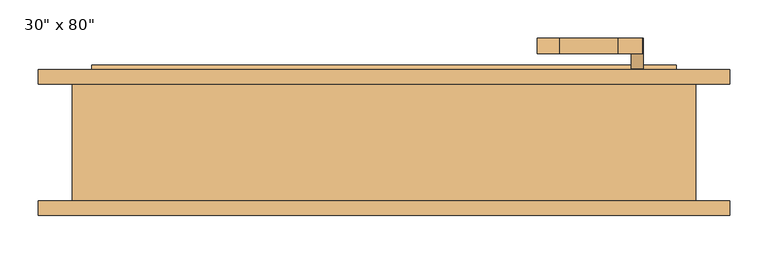
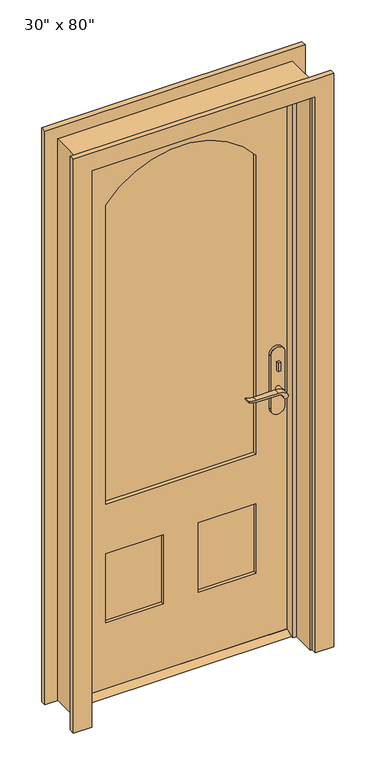
"""IFC4 building model written with IfcOpenShell, lengths in millimetres: door geometry."""

from ifc_helpers import new_model, si_unit, point, frame, frame_2d, origin, place, context, project, spatial, polyline, circle_curve, trimmed, segment, composite_curve, outline, extrude, faceted_brep, source, transform, mapped, element, save


def door_14b9be53(model_context):
    return source(origin(), model_context, "Body", "SolidModel", [
        extrude(outline(polyline([(38.1, 12.7), (73.025, 12.7), (98.425, 0.0), (12.7, 0.0), (38.1, 12.7)])), frame((-381.0, 0.0, 0.0), z_axis=(1.0, 0.0, 0.0), x_axis=(0.0, 1.0, 0.0)), (0.0, 0.0, 1.0), 762.0),
        extrude(outline(polyline([(335.2, 18.1), (325.2, 18.1), (325.2, 28.1), (335.2, 28.1), (335.2, 18.1)])), frame((0.0, 0.0, 981.9), z_axis=(0.0, 0.0, 1.0), x_axis=(1.0, 0.0, 0.0)), (0.0, 0.0, 1.0), 30.0),
        extrude(outline(composite_curve([segment(trimmed(circle_curve(frame_2d((996.9, 330.2)), 8.0), [point((996.9, 322.2))], [point((996.9, 338.2))], False, "CARTESIAN"), True, "CONTINUOUS"), segment(trimmed(circle_curve(frame_2d((996.9, 330.2)), 8.0), [point((996.9, 338.2))], [point((996.9, 322.2))], False, "CARTESIAN"), True, "CONTINUOUS")], self_intersect=False)), frame((0.0, 83.025, 0.0), z_axis=(0.0, 1.0, 0.0), x_axis=(0.0, 0.0, 1.0)), (0.0, 0.0, 1.0), 10.0),
        extrude(outline(composite_curve([segment(trimmed(circle_curve(frame_2d((897.1555521, 306.5324871)), 37.2832219), [point((919.0523287, 336.7081363))], [point((934.4, 304.8325667))], False, "CARTESIAN"), True, "CONTINUOUS"), segment(polyline([(934.4, 304.8325667), (934.4, 228.5564091)]), True, "CONTINUOUS"), segment(trimmed(circle_curve(frame_2d((1017.6850638, 228.6227909)), 83.2850902), [point((934.4, 228.5564091))], [point((939.4, 200.2))], True, "CARTESIAN"), True, "CONTINUOUS"), segment(polyline([(939.4, 200.2), (936.6135558, 200.2)]), True, "CONTINUOUS"), segment(trimmed(circle_curve(frame_2d((986.6709207, 232.1396612)), 59.3791355), [point((936.6135558, 200.2))], [point((927.4, 228.5564091))], False, "CARTESIAN"), True, "CONTINUOUS"), segment(polyline([(927.4, 228.5564091), (927.4, 304.8138099)]), True, "CONTINUOUS"), segment(trimmed(circle_curve(frame_2d((909.2738613, 304.8138099)), 18.1261387), [point((927.4, 304.8138099))], [point((914.4, 322.2))], True, "CARTESIAN"), True, "CONTINUOUS"), segment(trimmed(circle_curve(frame_2d((914.4, 330.2)), 8.0), [point((914.4, 322.2))], [point((919.0523287, 336.7081363))], False, "CARTESIAN"), True, "CONTINUOUS")], self_intersect=False)), frame((0.0, -21.9, 0.0), z_axis=(0.0, 1.0, 0.0), x_axis=(0.0, 0.0, 1.0)), (0.0, 0.0, 1.0), 20.0),
        extrude(outline(composite_curve([segment(trimmed(circle_curve(frame_2d((914.4, 330.2)), 8.0), [point((914.3999903, 322.2))], [point((919.0523287, 336.7081363))], False, "CARTESIAN"), True, "CONTINUOUS"), segment(trimmed(circle_curve(frame_2d((897.1555521, 306.5324871)), 37.2832219), [point((919.0523287, 336.7081363))], [point((934.4, 304.8325667))], False, "CARTESIAN"), True, "CONTINUOUS"), segment(polyline([(934.4, 304.8325667), (934.4, 228.5564091)]), True, "CONTINUOUS"), segment(trimmed(circle_curve(frame_2d((1017.6850638, 228.6227909)), 83.2850902), [point((934.4, 228.5564091))], [point((939.4, 200.2))], True, "CARTESIAN"), True, "CONTINUOUS"), segment(polyline([(939.4, 200.2), (936.6135558, 200.2)]), True, "CONTINUOUS"), segment(trimmed(circle_curve(frame_2d((986.6709207, 232.1396612)), 59.3791355), [point((936.6135558, 200.2))], [point((927.4, 228.5564091))], False, "CARTESIAN"), True, "CONTINUOUS"), segment(polyline([(927.4, 228.5564091), (927.4, 304.8138122)]), True, "CONTINUOUS"), segment(trimmed(circle_curve(frame_2d((909.2738682, 304.8138122)), 18.1261318), [point((927.4, 304.8138122))], [point((914.3999903, 322.2))], True, "CARTESIAN"), True, "CONTINUOUS")], self_intersect=False)), frame((0.0, 113.025, 0.0), z_axis=(0.0, 1.0, 0.0), x_axis=(0.0, 0.0, 1.0)), (0.0, 0.0, 1.0), 20.0),
        extrude(outline(composite_curve([segment(trimmed(circle_curve(frame_2d((914.4, 330.2)), 8.0), [point((914.4, 322.2))], [point((914.4, 338.2))], False, "CARTESIAN"), True, "CONTINUOUS"), segment(trimmed(circle_curve(frame_2d((914.4, 330.2)), 8.0), [point((914.4, 338.2))], [point((914.4, 322.2))], False, "CARTESIAN"), True, "CONTINUOUS")], self_intersect=False)), frame((0.0, -1.9, 0.0), z_axis=(0.0, 1.0, 0.0), x_axis=(0.0, 0.0, 1.0)), (0.0, 0.0, 1.0), 30.0),
        extrude(outline(composite_curve([segment(trimmed(circle_curve(frame_2d((914.4, 330.2)), 8.0), [point((914.4, 322.2))], [point((914.4, 338.2))], False, "CARTESIAN"), True, "CONTINUOUS"), segment(trimmed(circle_curve(frame_2d((914.4, 330.2)), 8.0), [point((914.4, 338.2))], [point((914.4, 322.2))], False, "CARTESIAN"), True, "CONTINUOUS")], self_intersect=False)), frame((0.0, 83.025, 0.0), z_axis=(0.0, 1.0, 0.0), x_axis=(0.0, 0.0, 1.0)), (0.0, 0.0, 1.0), 30.0),
        extrude(outline(composite_curve([segment(polyline([(844.4, 355.2), (1039.4, 355.2)]), True, "CONTINUOUS"), segment(trimmed(circle_curve(frame_2d((1039.4, 330.2)), 25.0), [point((1039.4, 355.2))], [point((1039.4, 305.2))], False, "CARTESIAN"), True, "CONTINUOUS"), segment(polyline([(1039.4, 305.2), (844.4, 305.2)]), True, "CONTINUOUS"), segment(trimmed(circle_curve(frame_2d((844.4, 330.2)), 25.0), [point((844.4, 305.2))], [point((844.4, 355.2))], False, "CARTESIAN"), True, "CONTINUOUS")], self_intersect=False)), frame((0.0, 28.1, 0.0), z_axis=(0.0, 1.0, 0.0), x_axis=(0.0, 0.0, 1.0)), (0.0, 0.0, 1.0), 10.0),
        extrude(outline(composite_curve([segment(polyline([(844.4, 355.2), (1039.4, 355.2)]), True, "CONTINUOUS"), segment(trimmed(circle_curve(frame_2d((1039.4, 330.2)), 25.0), [point((1039.4, 355.2))], [point((1039.4, 305.2))], False, "CARTESIAN"), True, "CONTINUOUS"), segment(polyline([(1039.4, 305.2), (844.4, 305.2)]), True, "CONTINUOUS"), segment(trimmed(circle_curve(frame_2d((844.4, 330.2)), 25.0), [point((844.4, 305.2))], [point((844.4, 355.2))], False, "CARTESIAN"), True, "CONTINUOUS")], self_intersect=False)), frame((0.0, 73.025, 0.0), z_axis=(0.0, 1.0, 0.0), x_axis=(0.0, 0.0, 1.0)), (0.0, 0.0, 1.0), 10.0),
        extrude(outline(polyline([(2032.0, -381.0), (12.7, -381.0), (12.7, 381.0), (2032.0, 381.0), (2032.0, -381.0)]), holes=[composite_curve([segment(polyline([(688.975, -260.35), (1784.35, -260.35)]), True, "CONTINUOUS"), segment(trimmed(circle_curve(frame_2d((1580.99125, 0.0)), 330.35875), [point((1784.35, -260.35))], [point((1784.35, 260.35))], True, "CARTESIAN"), True, "CONTINUOUS"), segment(polyline([(1784.35, 260.35), (688.975, 260.35), (688.975, -260.35)]), True, "CONTINUOUS")], self_intersect=False), polyline([(508.0, -60.325), (254.0, -60.325), (254.0, -260.35), (508.0, -260.35), (508.0, -60.325)]), polyline([(508.0, 260.35), (254.0, 260.35), (254.0, 60.325), (508.0, 60.325), (508.0, 260.35)])]), frame((0.0, 38.1, 0.0), z_axis=(0.0, 1.0, 0.0), x_axis=(0.0, 0.0, 1.0)), (0.0, 0.0, 1.0), 34.925),
        faceted_brep([(406.4, 73.025, 0.0), (406.4, -79.375, 0.0), (381.0, -79.375, 0.0), (381.0, 3.175, 0.0), (368.3, 3.175, 0.0), (368.3, 38.1, 0.0), (381.0, 38.1, 0.0), (381.0, 73.025, 0.0), (406.4, 73.025, 2057.4), (406.4, -79.375, 2057.4), (-406.4, -79.375, 2057.4), (-406.4, -79.375, 0.0), (-381.0, -79.375, 0.0), (-381.0, -79.375, 2032.0), (381.0, -79.375, 2032.0), (381.0, 3.175, 2032.0), (-381.0, 3.175, 2032.0), (-381.0, 3.175, 0.0), (-368.3, 3.175, 0.0), (-368.3, 3.175, 2019.3), (368.3, 3.175, 2019.3), (368.3, 38.1, 2019.3), (-368.3, 38.1, 2019.3), (-368.3, 38.1, 0.0), (-381.0, 38.1, 0.0), (-381.0, 38.1, 2032.0), (381.0, 38.1, 2032.0), (381.0, 73.025, 2032.0), (-381.0, 73.025, 2032.0), (-381.0, 73.025, 0.0), (-406.4, 73.025, 0.0), (-406.4, 73.025, 2057.4)], [[[0, 1, 2, 3, 4, 5, 6, 7]], [[1, 0, 8, 9]], [[2, 1, 9, 10, 11, 12, 13, 14]], [[3, 2, 14, 15]], [[4, 3, 15, 16, 17, 18, 19, 20]], [[5, 4, 20, 21]], [[6, 5, 21, 22, 23, 24, 25, 26]], [[7, 6, 26, 27]], [[0, 7, 27, 28, 29, 30, 31, 8]], [[9, 8, 31, 10]], [[15, 14, 13, 16]], [[21, 20, 19, 22]], [[27, 26, 25, 28]], [[30, 29, 24, 23, 18, 17, 12, 11]], [[10, 31, 30, 11]], [[16, 13, 12, 17]], [[22, 19, 18, 23]], [[28, 25, 24, 29]]]),
        extrude(outline(polyline([(-60.325, 49.7416667), (-260.35, 49.7416667), (-260.35, 61.3833333), (-60.325, 61.3833333), (-60.325, 49.7416667)])), frame((0.0, 0.0, 254.0), z_axis=(0.0, 0.0, 1.0), x_axis=(1.0, 0.0, 0.0)), (0.0, 0.0, 1.0), 254.0),
        extrude(outline(polyline([(260.35, 49.7416667), (60.325, 49.7416667), (60.325, 61.3833333), (260.35, 61.3833333), (260.35, 49.7416667)])), frame((0.0, 0.0, 254.0), z_axis=(0.0, 0.0, 1.0), x_axis=(1.0, 0.0, 0.0)), (0.0, 0.0, 1.0), 254.0),
        extrude(outline(composite_curve([segment(polyline([(688.975, -260.35), (688.975, 260.35), (1784.35, 260.35)]), True, "CONTINUOUS"), segment(trimmed(circle_curve(frame_2d((1580.99125, 0.0)), 330.35875), [point((1784.35, 260.35))], [point((1784.35, -260.35))], False, "CARTESIAN"), True, "CONTINUOUS"), segment(polyline([(1784.35, -260.35), (688.975, -260.35)]), True, "CONTINUOUS")], self_intersect=False)), frame((0.0, 52.07, 0.0), z_axis=(0.0, 1.0, 0.0), x_axis=(0.0, 0.0, 1.0)), (0.0, 0.0, 1.0), 6.985),
        extrude(outline(polyline([(0.0, -450.85), (0.0, -387.35), (2038.35, -387.35), (2038.35, 387.35), (0.0, 387.35), (0.0, 450.85), (2101.85, 450.85), (2101.85, -450.85), (0.0, -450.85)])), frame((0.0, -98.425, 0.0), z_axis=(0.0, 1.0, 0.0), x_axis=(0.0, 0.0, 1.0)), (0.0, 0.0, 1.0), 19.05),
        extrude(outline(polyline([(0.0, -450.85), (0.0, -387.35), (2038.35, -387.35), (2038.35, 387.35), (0.0, 387.35), (0.0, 450.85), (2101.85, 450.85), (2101.85, -450.85), (0.0, -450.85)])), frame((0.0, 73.025, 0.0), z_axis=(0.0, 1.0, 0.0), x_axis=(0.0, 0.0, 1.0)), (0.0, 0.0, 1.0), 19.05),
    ])


if __name__ == "__main__":
    model = new_model("IFC4")
    model_context = context("Model", 3, world=origin())
    ifc_project = project(units=[si_unit("LENGTHUNIT", "METRE", prefix="MILLI")], contexts=[model_context])
    site = spatial("IfcSite", under=ifc_project)
    building = spatial("IfcBuilding", under=site)
    placement = place(None, origin())
    door_shape = door_14b9be53(model_context)
    element("IfcDoor", 1, ObjectType="30\" x 80\"", at=placement, inside=building, context=model_context, shape_type="MappedRepresentation", body=[
        mapped(door_shape, transform((0.0, 0.0, 0.0), x_axis=(1.0, 0.0, 0.0), y_axis=(0.0, 1.0, 0.0), z_axis=(0.0, 0.0, 1.0))),
    ])
    save(model, "model.ifc")

# Revit data of these elements
# Type "30\" x 80\""
#   Type Mark = "8"
#   Assembly Code = "B2030100"
#   Analytic Construction = "French door, wood frame with single glass"
#   Threshold Offset [instance default] = 0' - 0 1/2"
#   Thickness = 0' - 1 3/8"
#   Thermal Resistance (R) = 1.0696 (h·ft²·°F)/BTU
#   Swing Angle [instance default] = 90.00°
#   Stiles = 0' - 4 3/4"
#   Rough Width = 2' - 8"
#   Rough Height = 6' - 9"
#   Radius = 1' - 1.00625"
#   Lock Rail = 0' - 7 1/8"
#   Height = 6' - 8"
#   Width = 2' - 6"
#   Heat Transfer Coefficient (U) = 0.9350 BTU/(h·ft²·°F)
#   Door Offset [instance default] = 0' - 0"
#   Bottom Rail = 0' - 9 1/2"
#   Threshold [instance default] = yes
#   Function = 1
#   Exterior Trim [instance default] = yes
#   Trim Material = Cherry
#   Threshold Material = Cherry
#   Panel Material = Cherry
#   Glazing = Glass
#   Frame Material = Cherry
#   Door Handle Material = Aluminum
#   Visual Light Transmittance = 0
#   Solar Heat Gain Coefficient = 0
#   Wall Closure = (empty or 0)
#   Construction Type = (empty or 0)
# Element 1 (IfcDoor, "30\" x 80\"")
#   Materials on its faces: "Cherry", "Aluminum", "Glass"
# Materials
#   "Cherry": class "Wood", colour RGB 226 177 128, transparency 0, Description = "Prunus Serotina", Cost = 0
#   "Glass": class "Glass", colour RGB 0 128 192, transparency 0.75, Description = "Soda Lime Glass", Cost = 0
#   "Aluminum": class "Metal", colour RGB 247 247 247, transparency 0, Description = "Aluminum 6061", Cost = 0
